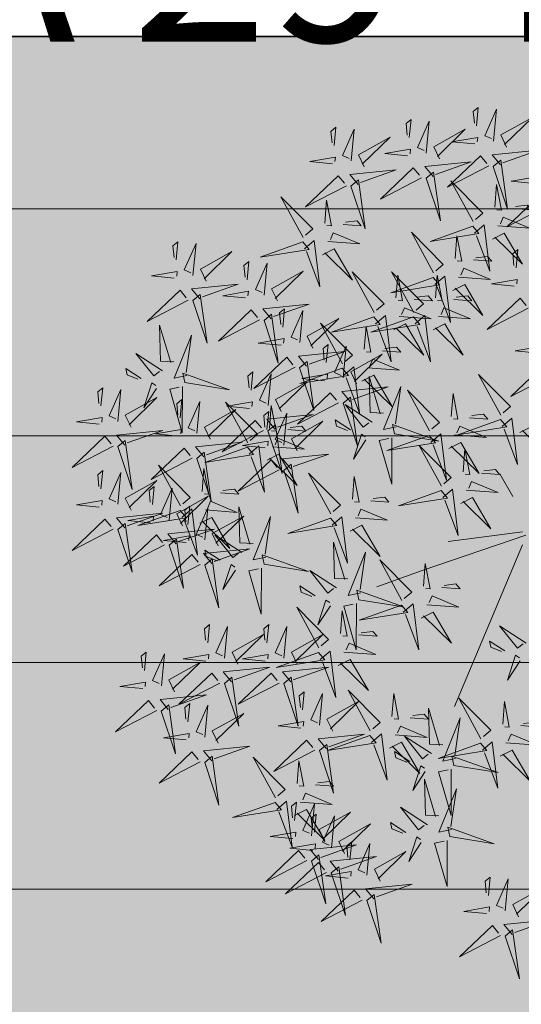
# Model space of a CAD drawing. Units: inches. Extents: x 1704 to 6393, y -157 to 1172.
# Tile 99 of 122: x 2561 to 2577, y 1001 to 1034. Entities that reach past the tile are written whole.
import ezdxf

# ---------------------------------------------------------------- set-up
doc = ezdxf.new("R2010")
doc.units = ezdxf.units.IN
doc.header["$MEASUREMENT"] = 0
for name, color, linetype, lineweight in [('A-ANNO-DIMS', 7, 'Continuous', 13), ('C-PROP', 7, 'Continuous', 35), ('L-DECK-PLNK-PATT', 250, 'Continuous', 13), ('L-shrub', 74, 'Continuous', 18), ('L-tree', 102, 'Continuous', 18)]:
    doc.layers.add(name, color=color, linetype=linetype, lineweight=lineweight)
doc.layers.add('L-DECK-PATT', color=35, linetype='Continuous', lineweight=13, true_color=0xa6725b)
doc.styles.get("Standard").update_dxf_attribs({"font": 'arial.ttf'})
doc.dimstyles.get("Standard").update_dxf_attribs({"dimtxt": 6, "dimasz": 2, "dimexe": 0.18, "dimexo": 0.0625, "dimgap": 0.09, "dimtad": 0, "dimtih": 1, "dimtoh": 1, "dimdec": 1, "dimzin": 0, "dimdsep": 46, "dimlunit": 3, "dimtxsty": 'Standard', "dimblk": 'ARCHTICK', "dimcen": 0.09, "dimadec": 0, "dimazin": 0, "dimtfac": 1, "dimtdec": 1, "dimtofl": 0, "dimtmove": 0, "dimatfit": 3, "dimfxl": 1, "dimtolj": 1, "dimtzin": 0, "dimarcsym": 0})

# ---------------------------------------------------------------- blocks, each defined once
blk = doc.blocks.new('bamboo')
blk.add_line((390, 162.3), (546.4, 218.1))
at = {"layer": 'L-shrub'}
for p, q in [((43.5, 73), (278.2, 631.2)), ((32.3, 39.5), (390, 162.3)), ((43.5, 28.4), (300.5, 61.9)), ((77, -94.4), (121.7, -172.6))]:
    blk.add_line(p, q, dxfattribs=at)
for points in [[(103.7, 1424.7), (54.4, 1572.3), (77.9, 1403.4), (103.7, 1424.7)], [(119.4, 1423.2), (261.4, 1496.7), (147.9, 1388.7), (126.6, 1414.5)], [(581.6, 1302), (532.2, 1449.6), (555.7, 1280.7), (581.6, 1302)], [(79.4, 1419.1), (107.8, 1384.6), (-52.4, 1368.4), (70.8, 1412)], [(597.3, 1300.4), (739.2, 1374), (625.7, 1265.9), (604.4, 1291.8)], [(57.7, 1357.7), (77.5, 1316.1), (-31.5, 1255.3), (64.8, 1349.1)], [(103.3, 1337.4), (92.8, 1227.4), (133.3, 1318.7), (110.4, 1328.8)], [(167.7, 1347.1), (246.3, 1339.5), (157.6, 1324.2), (159.1, 1340)], [(704.4, 1206.5), (655.1, 1354.1), (678.6, 1185.2), (704.4, 1206.5)], [(557.2, 1296.4), (585.7, 1261.9), (425.4, 1245.7), (548.6, 1289.3)], [(772.7, 1165.6), (723.3, 1313.2), (746.9, 1144.3), (772.7, 1165.6)], [(161.7, 1284.2), (155.7, 1221.3), (172.9, 1235.5), (168.8, 1275.6)], [(720.2, 1205), (862.1, 1278.5), (748.6, 1170.5), (727.3, 1196.4)], [(303.5, 1094), (304.2, 1253.9), (347.3, 1103.2), (314.4, 1096.3)], [(535.5, 1235), (555.3, 1193.4), (446.4, 1132.5), (542.6, 1226.4)], [(788.4, 1164.1), (930.3, 1237.6), (816.9, 1129.6), (795.5, 1155.5)], [(680.1, 1200.9), (708.6, 1166.4), (548.3, 1150.2), (671.5, 1193.8)], [(581.2, 1214.7), (570.7, 1104.6), (611.1, 1195.9), (588.3, 1206.1)], [(645.6, 1224.3), (724.2, 1216.7), (635.4, 1201.5), (637, 1217.2)], [(393.3, 1101.5), (436.5, 1167.6), (408.8, 1082), (395.6, 1090.6)], [(748.4, 1160), (776.8, 1125.5), (616.6, 1109.3), (739.8, 1152.9)], [(639.6, 1161.5), (633.5, 1098.6), (650.8, 1112.8), (646.7, 1152.8)], [(658.4, 1139.6), (678.2, 1098), (569.2, 1037.1), (665.5, 1130.9)], [(768.4, 1128.9), (847.1, 1121.3), (758.3, 1106.1), (759.8, 1121.8)], [(294.9, 1080.8), (141.2, 1105.5), (301.8, 1048), (294.9, 1080.8)], [(726.6, 1098.6), (746.5, 1057), (637.5, 996.2), (733.8, 1090)], [(704, 1119.3), (693.5, 1009.2), (734, 1100.5), (711.2, 1110.6)], [(830.7, 1007.8), (789.5, 987.1), (726.4, 1094.8), (822.2, 1000.5)], [(892.5, 987.3), (858.6, 958.2), (839.1, 1118), (885.2, 995.8)], [(288.5, 1056.7), (332.3, 1065.9), (272.3, 916.4), (290.8, 1045.7)], [(372, 1040), (464.6, 979.6), (402.5, 1057.8), (382.9, 1042.3)], [(446.2, 1067), (499.2, 1032.5), (494.6, 1054.4), (457.2, 1069.3)], [(762.4, 1066), (756.4, 1003.1), (773.6, 1017.3), (769.5, 1057.4)], [(772.3, 1078.4), (761.8, 968.3), (802.3, 1059.6), (779.4, 1069.7)], [(836.7, 1088), (915.3, 1080.4), (826.6, 1065.2), (828.1, 1080.9)], [(830.7, 1025.1), (824.7, 962.2), (841.9, 976.4), (837.8, 1016.5)], [(289.9, 848.6), (290.5, 1008.4), (333.6, 857.8), (300.8, 850.9)], [(332.8, 1008.9), (378.9, 1007.2), (382.3, 882.5), (343.8, 1011.2)], [(898.5, 963.1), (1045.1, 1015.5), (876.7, 988.5), (898.5, 963.1)], [(811.3, 961.7), (701, 970), (793.1, 931.4), (802.8, 954.4)], [(1141.3, 824.7), (1092, 972.3), (1115.5, 803.4), (1141.3, 824.7)], [(379.6, 856.1), (422.9, 922.2), (395.2, 836.5), (381.9, 845.1)], [(745.4, 783.8), (696, 931.4), (719.6, 762.5), (745.4, 783.8)], [(897.3, 947.3), (973.8, 807), (863.4, 918.2), (888.9, 940.1)], [(120.7, 803.3), (79.5, 782.6), (16.5, 890.3), (112.2, 796)], [(182.5, 782.8), (148.6, 753.6), (129.1, 913.5), (175.2, 791.2)], [(564.8, 755.5), (530.9, 726.4), (511.4, 886.2), (557.5, 764)], [(759.2, 902.3), (696.2, 907), (710.8, 890.1), (750.8, 895)], [(822.2, 897.5), (816.2, 818.8), (799.2, 907.2), (815, 906)], [(1157.1, 823.2), (1299, 896.7), (1185.5, 788.7), (1164.2, 814.6)], [(281.2, 835.4), (127.5, 860.1), (288.1, 802.6), (281.2, 835.4)], [(503, 776), (461.8, 755.3), (398.7, 863), (494.5, 768.7)], [(761.1, 782.3), (903, 855.8), (789.6, 747.8), (768.2, 773.7)], [(274.9, 811.2), (318.6, 820.4), (258.7, 670.9), (277.2, 800.3)], [(432.6, 821.6), (485.5, 787.1), (480.9, 808.9), (443.5, 823.9)], [(1117, 819.1), (1145.4, 784.6), (985.2, 768.4), (1108.4, 812)], [(188.6, 758.6), (335.2, 810.9), (166.8, 784), (188.6, 758.6)], [(358.3, 794.5), (451, 734.2), (388.8, 812.4), (369.3, 796.8)], [(570.9, 731.3), (717.4, 783.7), (549, 756.7), (570.9, 731.3)], [(1291.5, 647.4), (1242.1, 795), (1265.7, 626.1), (1291.5, 647.4)], [(101.4, 757.2), (-8.9, 765.5), (83.2, 726.9), (92.9, 749.9)], [(319.2, 763.5), (365.2, 761.8), (368.6, 637), (330.1, 765.8)], [(721.1, 778.2), (749.5, 743.7), (589.3, 727.5), (712.5, 771.1)], [(1095.3, 757.7), (1115.1, 716.2), (1006.1, 655.3), (1102.4, 749.1)], [(187.4, 742.8), (263.8, 602.4), (153.5, 713.7), (178.9, 735.5)], [(483.6, 729.9), (373.4, 738.2), (465.5, 699.6), (475.2, 722.6)], [(569.7, 715.5), (646.1, 575.2), (535.8, 686.4), (561.2, 708.3)], [(699.3, 716.8), (719.2, 675.2), (610.2, 614.4), (706.4, 708.2)], [(1140.9, 737.5), (1130.4, 627.4), (1170.9, 718.7), (1148, 728.8)], [(1205.3, 747.1), (1283.9, 739.5), (1195.2, 724.3), (1196.7, 740)], [(1307.2, 645.9), (1449.1, 719.5), (1335.7, 611.4), (1314.3, 637.3)], [(49.3, 697.7), (-13.7, 702.5), (0.8, 685.5), (40.8, 690.4)], [(112.3, 693), (106.3, 614.2), (89.3, 702.6), (105, 701.5)], [(745, 696.6), (734.5, 586.5), (774.9, 677.8), (752.1, 687.9)], [(809.4, 706.2), (888, 698.6), (799.3, 683.4), (800.8, 699.1)], [(868.3, 552), (818.9, 699.6), (842.4, 530.7), (868.3, 552)], [(1073.1, 552), (1023.7, 699.6), (1047.2, 530.7), (1073.1, 552)], [(1199.3, 684.2), (1193.3, 621.3), (1210.5, 635.5), (1206.4, 675.6)], [(431.6, 670.5), (368.6, 675.2), (383.1, 658.2), (423.1, 663.2)], [(494.6, 665.7), (488.6, 587), (471.6, 675.4), (487.3, 674.2)], [(803.4, 643.3), (797.4, 580.4), (814.6, 594.6), (810.5, 634.7)], [(884, 550.5), (1025.9, 624), (912.4, 516), (891.1, 541.8)], [(1088.8, 550.5), (1230.7, 624), (1117.2, 516), (1095.9, 541.8)], [(1267.2, 641.9), (1295.6, 607.4), (1135.4, 591.1), (1258.6, 634.8)], [(742.3, 469.2), (708.4, 440), (688.9, 599.9), (735, 477.6)], [(1245.4, 580.5), (1265.3, 538.9), (1156.3, 478), (1252.6, 571.9)], [(680.5, 489.6), (639.3, 469), (576.2, 576.7), (672, 482.3)], [(843.9, 546.4), (872.4, 511.9), (712.1, 495.7), (835.3, 539.3)], [(1048.7, 546.4), (1077.2, 511.9), (916.9, 495.7), (1040.1, 539.3)], [(1291.1, 560.2), (1280.6, 450.1), (1321.1, 541.4), (1298.2, 551.6)], [(1355.5, 569.8), (1434.1, 562.2), (1345.4, 547), (1346.9, 562.7)], [(52, 474.3), (95.2, 540.4), (67.5, 454.7), (54.3, 463.3)], [(748.4, 444.9), (894.9, 497.3), (726.5, 470.3), (748.4, 444.9)], [(822.2, 485), (842, 443.4), (733.1, 382.6), (829.3, 476.4)], [(1027, 485), (1046.8, 443.4), (937.9, 382.6), (1034.1, 476.4)], [(1349.5, 506.9), (1343.5, 444), (1360.7, 458.2), (1356.6, 498.3)], [(661.1, 443.6), (550.9, 451.8), (643, 413.2), (652.6, 436.3)], [(867.9, 464.7), (857.4, 354.7), (897.8, 446), (875, 456.1)], [(932.3, 474.4), (1010.9, 466.8), (922.2, 451.6), (923.7, 467.3)], [(1072.7, 464.7), (1062.1, 354.7), (1102.6, 446), (1079.8, 456.1)], [(1137.1, 474.4), (1215.7, 466.8), (1126.9, 451.6), (1128.4, 467.3)], [(30.7, 412.7), (123.3, 352.4), (61.2, 430.6), (41.6, 415)], [(104.9, 439.8), (157.9, 405.3), (153.3, 427.1), (115.9, 442.1)], [(393.8, 326), (352.6, 305.3), (289.5, 413), (385.3, 318.7)], [(455.6, 305.5), (421.7, 276.4), (402.2, 436.3), (448.3, 314)], [(617.5, 275.9), (618.2, 435.7), (661.3, 285.1), (628.5, 278.2)], [(747.2, 429.2), (823.6, 288.8), (713.3, 400), (738.7, 421.9)], [(926.3, 411.5), (920.3, 348.6), (937.5, 362.8), (933.4, 402.9)], [(1131.1, 411.5), (1125, 348.6), (1142.3, 362.8), (1138.2, 402.9)], [(609.1, 384.1), (546.1, 388.8), (560.6, 371.9), (600.6, 376.8)], [(672.1, 379.4), (666.1, 300.6), (649, 389), (664.8, 387.8)], [(707.3, 283.4), (750.5, 349.5), (722.8, 263.8), (709.6, 272.4)], [(461.7, 281.3), (608.2, 333.7), (439.8, 306.7), (461.7, 281.3)], [(945.2, 153.2), (945.8, 313), (988.9, 162.4), (956.1, 155.5)], [(374.4, 279.9), (264.1, 288.2), (356.3, 249.6), (365.9, 272.6)], [(608.9, 262.7), (455.2, 287.4), (615.8, 229.9), (608.9, 262.7)], [(1141.3, 142.9), (1092, 290.5), (1115.5, 121.6), (1141.3, 142.9)], [(460.4, 265.6), (536.9, 125.2), (426.5, 236.4), (452, 258.3)], [(602.5, 238.5), (646.3, 247.7), (586.3, 98.2), (604.8, 227.6)], [(686, 221.8), (778.6, 161.5), (716.5, 239.7), (696.9, 224.1)], [(760.2, 248.9), (813.2, 214.4), (808.6, 236.2), (771.2, 251.2)], [(322.4, 220.5), (259.3, 225.2), (273.9, 208.3), (313.9, 213.2)], [(385.4, 215.7), (379.4, 137), (362.3, 225.4), (378.1, 224.2)], [(1035, 160.6), (1078.2, 226.8), (1050.5, 141.1), (1037.3, 149.7)], [(1157.1, 141.4), (1299, 214.9), (1185.5, 106.9), (1164.2, 132.8)], [(1264.2, 74.7), (1214.8, 222.3), (1238.4, 53.4), (1264.2, 74.7)], [(646.8, 190.8), (692.9, 189.1), (696.3, 64.3), (657.8, 193.1)], [(701.3, 5.5), (667.4, -23.6), (647.9, 136.3), (694, 14)], [(936.5, 139.9), (782.9, 164.7), (943.4, 107.2), (936.5, 139.9)], [(1117, 137.3), (1145.4, 102.8), (985.2, 86.6), (1108.4, 130.2)], [(1279.9, 73.2), (1421.8, 146.8), (1308.4, 38.7), (1287, 64.6)], [(1441.7, 20.2), (1392.3, 167.8), (1415.9, -1.1), (1441.7, 20.2)], [(639.5, 26), (598.3, 5.3), (535.3, 113), (631, 18.7)], [(930.2, 115.8), (973.9, 125), (914, -24.5), (932.5, 104.9)], [(1013.6, 99.1), (1106.3, 38.8), (1044.2, 116.9), (1024.6, 101.4)], [(1087.9, 126.1), (1140.9, 91.6), (1136.3, 113.5), (1098.9, 128.4)], [(1220.1, -21.7), (1186.2, -50.9), (1166.7, 109), (1212.8, -13.3)], [(974.5, 68.1), (1020.5, 66.3), (1023.9, -58.4), (985.4, 70.4)], [(1095.3, 76), (1115.1, 34.4), (1006.1, -26.5), (1102.4, 67.3)], [(1158.3, -1.3), (1117.1, -21.9), (1054.1, 85.8), (1149.8, -8.5)], [(1239.9, 69.2), (1268.3, 34.7), (1108.1, 18.4), (1231.3, 62.1)], [(1457.4, 18.7), (1599.3, 92.2), (1485.9, -15.8), (1464.5, 10)], [(319, -89.9), (285.1, -119.1), (265.6, 40.8), (311.8, -81.4)], [(1140.9, 55.7), (1130.4, -54.4), (1170.9, 36.9), (1148, 47)], [(1205.3, 65.3), (1283.9, 57.7), (1195.2, 42.5), (1196.7, 58.2)], [(257.2, -69.4), (216.1, -90.1), (153, 17.6), (248.8, -76.7)], [(707.4, -18.7), (854, 33.7), (685.6, 6.7), (707.4, -18.7)], [(1218.1, 7.8), (1238, -33.8), (1129, -94.7), (1225.2, -0.8)], [(1199.3, 2.4), (1193.3, -60.5), (1210.5, -46.3), (1206.4, -6.2)], [(1226.2, -46), (1372.8, 6.4), (1204.4, -20.6), (1226.2, -46)], [(1417.4, 14.6), (1445.8, -19.9), (1285.6, -36.1), (1408.7, 7.5)], [(620.2, -20.1), (509.9, -11.8), (602, -50.4), (611.7, -27.3)], [(1263.8, -12.5), (1253.3, -122.6), (1293.7, -31.3), (1270.9, -21.1)], [(1328.2, -2.9), (1406.8, -10.5), (1318.1, -25.7), (1319.6, -10)], [(325.1, -114.1), (471.7, -61.8), (303.3, -88.7), (325.1, -114.1)], [(706.2, -34.4), (782.6, -174.8), (672.3, -63.6), (697.7, -41.7)], [(868.3, -184.3), (818.9, -36.7), (842.4, -205.6), (868.3, -184.3)], [(1139, -47.3), (1028.7, -39.1), (1120.8, -77.6), (1130.5, -54.6)], [(1225, -61.7), (1301.4, -202.1), (1191.1, -90.8), (1216.5, -69)], [(1395.6, -46.8), (1415.5, -88.4), (1306.5, -149.2), (1402.7, -55.4)], [(1322.2, -65.8), (1316.2, -128.7), (1333.4, -114.5), (1329.3, -74.4)], [(1441.3, -67.1), (1430.8, -177.1), (1471.2, -85.8), (1448.4, -75.7)], [(1505.7, -57.4), (1584.3, -65), (1495.6, -80.2), (1497.1, -64.5)], [(568.1, -79.5), (505.1, -74.8), (519.6, -91.7), (559.6, -86.8)], [(631.1, -84.2), (625.1, -163), (608.1, -74.6), (623.8, -75.8)], [(1168.6, -225.3), (1119.3, -77.6), (1142.8, -246.6), (1168.6, -225.3)], [(1149.9, -111.5), (1143.9, -190.3), (1126.9, -101.9), (1142.6, -103)], [(237.9, -115.5), (127.6, -107.2), (219.7, -145.8), (229.4, -122.8)], [(323.9, -129.9), (400.4, -270.3), (290, -159), (315.4, -137.2)], [(926.2, -219.4), (885, -240.1), (822, -132.4), (917.7, -226.7)], [(884, -185.9), (1025.9, -112.3), (912.4, -220.4), (891.1, -194.5)], [(988, -239.9), (954.1, -269), (934.6, -109.2), (980.8, -231.4)], [(1086.9, -106.8), (1023.9, -102.1), (1038.4, -119), (1078.4, -114.1)], [(1441.7, -266.2), (1392.3, -118.6), (1415.9, -287.5), (1441.7, -266.2)], [(1499.7, -120.3), (1493.7, -183.2), (1510.9, -169), (1506.8, -128.9)], [(248.8, -179.7), (242.8, -258.4), (225.8, -170), (241.6, -171.2)], [(360, -280.8), (326.1, -310), (306.6, -150.1), (352.7, -272.3)], [(494.6, -296.8), (495.3, -137), (538.4, -287.6), (505.6, -294.5)], [(1184.4, -226.8), (1326.3, -153.2), (1212.8, -261.3), (1191.5, -235.4)], [(185.8, -175), (122.8, -170.2), (137.4, -187.2), (177.4, -182.3)], [(298.2, -260.3), (257, -281), (193.9, -173.3), (289.7, -267.6)], [(843.9, -189.9), (872.4, -224.4), (712.1, -240.6), (835.3, -197)], [(922.9, -320.7), (873.5, -173.1), (897.1, -342), (922.9, -320.7)], [(1457.4, -267.7), (1599.3, -194.1), (1485.9, -302.2), (1464.5, -276.3)], [(52.5, -314.9), (11.3, -335.6), (-51.8, -227.9), (44, -322.2)], [(114.3, -335.4), (80.4, -364.5), (60.9, -204.6), (107, -326.9)], [(584.4, -289.3), (627.6, -223.2), (600, -308.9), (586.7, -300.3)], [(994.1, -264.1), (1140.7, -211.8), (972.3, -238.7), (994.1, -264.1)], [(1144.3, -230.8), (1172.7, -265.3), (1012.5, -281.6), (1135.7, -237.9)], [(366.1, -305), (512.7, -252.7), (344.3, -279.6), (366.1, -305)], [(663.5, -416.2), (614.1, -268.5), (637.6, -437.5), (663.5, -416.2)], [(822.2, -251.3), (842, -292.9), (733.1, -353.8), (829.3, -259.9)], [(906.9, -265.5), (796.6, -257.2), (888.7, -295.8), (898.4, -272.8)], [(867.9, -271.6), (857.4, -381.7), (897.8, -290.4), (875, -280.2)], [(932.3, -262), (1010.9, -269.6), (922.2, -284.8), (923.7, -269.1)], [(938.6, -322.2), (1080.5, -248.7), (967.1, -356.7), (945.7, -330.8)], [(1417.4, -271.7), (1445.8, -306.2), (1285.6, -322.5), (1408.7, -278.8)], [(278.8, -306.4), (168.6, -298.1), (260.7, -336.7), (270.4, -313.7)], [(486, -310), (332.3, -285.3), (492.9, -342.8), (486, -310)], [(992.9, -279.9), (1069.3, -420.3), (959, -309), (984.4, -287.2)], [(1122.6, -292.2), (1142.4, -333.8), (1033.4, -394.7), (1129.7, -300.8)], [(1232.6, -302.9), (1311.2, -310.5), (1222.5, -325.7), (1224, -310)], [(120.3, -359.6), (266.9, -307.2), (98.5, -334.2), (120.3, -359.6)], [(364.9, -320.8), (441.3, -461.2), (331, -349.9), (356.4, -328.1)], [(479.7, -334.2), (523.4, -325), (463.5, -474.5), (482, -345.1)], [(563.1, -350.9), (655.8, -411.2), (593.6, -333), (574, -348.6)], [(637.4, -323.8), (690.3, -358.3), (685.7, -336.5), (648.3, -321.5)], [(898.6, -326.3), (927, -360.8), (766.8, -377), (889.9, -333.4)], [(854.8, -325), (791.8, -320.2), (806.4, -337.2), (846.3, -332.2)], [(917.8, -329.7), (911.8, -408.4), (894.8, -320), (910.5, -321.2)], [(926.3, -324.9), (920.3, -387.8), (937.5, -373.5), (933.4, -333.5)], [(1168.2, -312.5), (1157.7, -422.6), (1198.2, -331.3), (1175.3, -321.1)], [(1218.2, -474.1), (1218.9, -314.2), (1262, -464.9), (1229.2, -471.8)], [(1395.6, -333.1), (1415.5, -374.7), (1306.5, -435.6), (1402.7, -341.7)], [(226.8, -365.9), (163.8, -361.1), (178.3, -378.1), (218.3, -373.2)], [(289.8, -370.6), (283.8, -449.3), (266.8, -360.9), (282.5, -362.1)], [(679.2, -417.7), (821.1, -344.1), (707.7, -452.2), (686.3, -426.3)], [(1226.6, -365.8), (1220.6, -428.7), (1237.8, -414.5), (1233.7, -374.4)], [(1441.3, -353.4), (1430.8, -463.5), (1471.2, -372.2), (1448.4, -362)], [(1505.7, -343.8), (1584.3, -351.4), (1495.6, -366.6), (1497.1, -350.9)], [(119.1, -375.3), (195.6, -515.7), (85.2, -404.5), (110.7, -382.6)], [(598.6, -492.1), (557.4, -512.8), (494.3, -405.1), (590.1, -499.4)], [(524, -381.9), (570, -383.6), (573.4, -508.4), (534.9, -379.6)], [(660.4, -512.6), (626.5, -541.8), (607, -381.9), (653.1, -504.2)], [(813.7, -538.9), (764.3, -391.3), (787.8, -560.2), (813.7, -538.9)], [(876.8, -387.7), (896.6, -429.3), (787.7, -490.1), (883.9, -396.3)], [(922.5, -407.9), (912, -518), (952.4, -426.7), (929.6, -416.6)], [(986.9, -398.3), (1065.5, -405.9), (976.8, -421.1), (978.3, -405.4)], [(1308, -466.6), (1351.2, -400.5), (1323.6, -486.2), (1310.3, -477.5)], [(1499.7, -406.7), (1493.7, -469.6), (1510.9, -455.4), (1506.8, -415.3)], [(-58, -513.1), (83.9, -439.6), (-29.6, -547.6), (-50.9, -521.7)], [(639.2, -421.7), (667.6, -456.2), (507.4, -472.5), (630.5, -428.8)], [(829.4, -540.4), (971.3, -466.8), (857.8, -574.9), (836.5, -549)], [(980.9, -461.2), (974.9, -524.1), (992.1, -509.9), (988, -469.8)], [(1209.6, -487.3), (1055.9, -462.6), (1216.5, -520.1), (1209.6, -487.3)], [(617.4, -483.1), (637.2, -524.7), (528.3, -585.6), (624.5, -491.7)], [(666.4, -536.8), (813, -484.5), (644.6, -511.4), (666.4, -536.8)], [(663.1, -503.4), (652.6, -613.5), (693, -522.2), (670.2, -512)], [(727.5, -493.8), (806.1, -501.4), (717.4, -516.6), (718.9, -500.9)], [(1203.3, -511.5), (1247, -502.3), (1187.1, -651.7), (1205.5, -522.4)], [(1361, -501.1), (1413.9, -535.6), (1409.3, -513.8), (1371.9, -498.8)], [(579.2, -538.2), (468.9, -529.9), (561.1, -568.5), (570.7, -545.5)], [(1286.7, -528.1), (1379.3, -588.5), (1317.2, -510.3), (1297.6, -525.8)], [(414.6, -689.9), (380.7, -719), (361.2, -559.2), (407.3, -681.4)], [(551.1, -689.9), (517.2, -719), (497.7, -559.2), (543.9, -681.4)], [(665.2, -552.6), (741.7, -693), (631.3, -581.7), (656.8, -559.9)], [(789.3, -544.5), (817.8, -578.9), (657.5, -595.2), (780.7, -551.6)], [(721.5, -556.7), (715.5, -619.6), (732.7, -605.4), (728.6, -565.3)], [(936.5, -702.5), (887.2, -554.9), (910.7, -723.8), (936.5, -702.5)], [(1247.5, -559.2), (1293.6, -560.9), (1297, -685.7), (1258.5, -556.9)], [(-9.8, -589.2), (68.8, -596.8), (-19.9, -612), (-18.4, -596.3)], [(352.8, -669.4), (311.6, -690.1), (248.5, -582.4), (344.3, -676.7)], [(489.3, -669.4), (448.2, -690.1), (385.1, -582.4), (480.9, -676.7)], [(527.1, -597.7), (464.1, -593), (478.7, -609.9), (518.7, -605)], [(590.2, -602.4), (584.1, -681.2), (567.1, -592.8), (582.9, -593.9)], [(767.6, -605.8), (787.4, -647.4), (678.5, -708.3), (774.7, -614.5)], [(813.3, -626.1), (802.7, -736.2), (843.2, -644.9), (820.4, -634.7)], [(877.7, -616.5), (956.3, -624.1), (867.5, -639.3), (869, -623.6)], [(952.3, -704), (1094.2, -630.5), (980.7, -738.5), (959.4, -712.7)], [(1182.3, -770.7), (1132.9, -623.1), (1156.5, -792), (1182.3, -770.7)], [(23.9, -744.9), (165.8, -671.4), (52.3, -779.4), (31, -753.6)], [(420.7, -714.1), (567.3, -661.7), (398.9, -688.7), (420.7, -714.1)], [(557.2, -714.1), (703.8, -661.7), (535.4, -688.7), (557.2, -714.1)], [(871.6, -679.4), (865.6, -742.3), (882.9, -728.1), (878.8, -688)], [(333.5, -715.5), (223.2, -707.2), (315.3, -745.8), (325, -722.8)], [(346.4, -826.2), (312.4, -855.4), (293, -695.5), (339.1, -817.8)], [(470, -715.5), (359.7, -707.2), (451.8, -745.8), (461.5, -722.8)], [(912.2, -708.1), (940.6, -742.6), (780.4, -758.8), (903.6, -715.2)], [(1198, -772.2), (1339.9, -698.7), (1226.5, -806.7), (1205.1, -780.8)], [(284.5, -805.8), (243.4, -826.4), (180.3, -718.7), (276.1, -813.1)], [(419.5, -729.9), (495.9, -870.2), (385.6, -759), (411, -737.1)], [(556, -729.9), (632.4, -870.2), (522.1, -759), (547.5, -737.1)], [(281.4, -774.9), (218.4, -770.2), (232.9, -787.1), (272.9, -782.2)], [(344.4, -779.7), (338.4, -858.4), (321.4, -770), (337.1, -771.2)], [(417.9, -774.9), (354.9, -770.2), (369.5, -787.1), (409.4, -782.2)], [(480.9, -779.7), (474.9, -858.4), (457.9, -770), (473.7, -771.2)], [(890.5, -769.5), (910.3, -811.1), (801.3, -871.9), (897.6, -778.1)], [(1000.5, -780.1), (1079.1, -787.7), (990.4, -802.9), (991.9, -787.2)], [(1158, -776.3), (1186.4, -810.8), (1026.2, -827), (1149.3, -783.4)], [(352.4, -850.5), (499, -798.1), (330.6, -825.1), (352.4, -850.5)], [(936.1, -789.8), (925.6, -899.8), (966.1, -808.5), (943.2, -798.4)], [(72.2, -821), (150.8, -828.6), (62, -843.8), (63.5, -828.1)], [(265.2, -851.8), (154.9, -843.6), (247, -882.2), (256.7, -859.1)], [(735.1, -928.5), (693.9, -949.2), (630.8, -841.5), (726.6, -935.8)], [(796.9, -949), (763, -978.1), (743.5, -818.2), (789.6, -940.5)], [(994.5, -843), (988.5, -905.9), (1005.7, -891.7), (1001.6, -851.6)], [(1136.2, -837.6), (1156, -879.2), (1047.1, -940.1), (1143.3, -846.3)], [(1246.3, -848.3), (1324.9, -855.9), (1236.2, -871.1), (1237.7, -855.4)], [(66.1, -883.9), (60.1, -946.8), (77.4, -932.6), (73.3, -892.5)], [(209.8, -1003.5), (175.9, -1032.7), (156.4, -872.8), (202.6, -995)], [(351.2, -866.2), (427.7, -1006.6), (317.3, -895.4), (342.8, -873.5)], [(1181.9, -857.9), (1171.4, -968), (1211.8, -876.7), (1189, -866.6)], [(148, -983), (106.8, -1003.7), (43.8, -896), (139.5, -990.3)], [(213.1, -911.3), (150.1, -906.6), (164.7, -923.5), (204.7, -918.6)], [(276.1, -916), (270.1, -994.8), (253.1, -906.4), (268.9, -907.6)], [(1240.3, -911.2), (1234.3, -974.1), (1251.5, -959.9), (1247.4, -919.8)], [(803, -973.2), (949.5, -920.8), (781.1, -947.8), (803, -973.2)], [(215.9, -1027.7), (362.5, -975.4), (194.1, -1002.3), (215.9, -1027.7)], [(715.7, -974.6), (605.5, -966.3), (697.6, -1004.9), (707.3, -981.8)], [(636.2, -1166.1), (586.8, -1018.5), (610.3, -1187.4), (636.2, -1166.1)], [(801.8, -988.9), (878.2, -1129.3), (767.9, -1018.1), (793.3, -996.2)], [(-44.4, -1099.5), (97.5, -1025.9), (-15.9, -1134), (-37.3, -1108.1)], [(128.7, -1029.1), (18.4, -1020.8), (110.5, -1059.4), (120.2, -1036.4)], [(214.7, -1043.5), (291.1, -1183.9), (180.8, -1072.6), (206.2, -1050.8)], [(376.8, -1193.4), (327.4, -1045.8), (350.9, -1214.7), (376.8, -1193.4)], [(663.7, -1034), (600.7, -1029.3), (615.2, -1046.2), (655.2, -1041.3)], [(726.7, -1038.7), (720.7, -1117.5), (703.7, -1029.1), (719.4, -1030.3)], [(76.6, -1088.6), (13.6, -1083.8), (28.1, -1100.8), (68.1, -1095.8)], [(144.7, -1234.3), (95.3, -1086.7), (118.8, -1255.6), (144.7, -1234.3)], [(139.6, -1093.3), (133.6, -1172), (116.6, -1083.6), (132.3, -1084.8)], [(392.5, -1194.9), (534.4, -1121.4), (420.9, -1229.4), (399.6, -1203.5)], [(651.9, -1167.6), (793.8, -1094.1), (680.3, -1202.1), (659, -1176.3)], [(3.9, -1175.6), (82.5, -1183.2), (-6.2, -1198.4), (-4.7, -1182.7)], [(160.4, -1235.8), (302.3, -1162.3), (188.8, -1270.3), (167.5, -1244.4)], [(611.8, -1171.7), (640.3, -1206.2), (480.1, -1222.4), (603.2, -1178.8)], [(352.4, -1199), (380.9, -1233.5), (220.7, -1249.7), (343.8, -1206.1)], [(120.3, -1239.9), (148.8, -1274.4), (-11.4, -1290.6), (111.7, -1247)], [(590.1, -1233.1), (609.9, -1274.7), (501, -1335.5), (597.2, -1241.7)], [(635.8, -1253.4), (625.3, -1363.4), (665.7, -1272.1), (642.9, -1262)], [(700.2, -1243.7), (778.8, -1251.3), (690.1, -1266.6), (691.6, -1250.8)], [(330.7, -1260.4), (350.5, -1301.9), (241.6, -1362.8), (337.8, -1269)], [(376.4, -1280.6), (365.9, -1390.7), (406.3, -1299.4), (383.5, -1289.3)], [(440.8, -1271), (519.4, -1278.6), (430.7, -1293.8), (432.2, -1278.1)], [(98.6, -1301.3), (118.4, -1342.9), (9.5, -1403.7), (105.7, -1309.9)], [(144.3, -1321.5), (133.8, -1431.6), (174.2, -1340.3), (151.4, -1330.2)], [(208.7, -1311.9), (287.3, -1319.5), (198.6, -1334.7), (200.1, -1319)], [(694.2, -1306.6), (688.2, -1369.5), (705.4, -1355.3), (701.3, -1315.3)], [(434.8, -1333.9), (428.8, -1396.8), (446, -1382.6), (441.9, -1342.5)], [(202.7, -1374.8), (196.7, -1437.7), (213.9, -1423.5), (209.8, -1383.4)]]:
    blk.add_lwpolyline(points, dxfattribs=at)
blk = doc.blocks.new('_ArchTick')
at = {"color": 0, "linetype": 'ByBlock', "const_width": 0.15}
blk.add_lwpolyline([(-0.5, -0.5), (0.5, 0.5)], dxfattribs=at)
blk = doc.blocks.new('*D88')
at = {"layer": 'A-ANNO-DIMS', "color": 0, "lineweight": -2, "transparency": 16777216}
for p, q in [((2596.639, 1031.77), (2596.639, 1036.222)), ((2625.54, 1031.77), (2625.54, 1036.222)), ((2596.639, 1036.042), (2594.639, 1036.042)), ((2625.54, 1036.042), (2596.639, 1036.042))]:
    blk.add_line(p, q, dxfattribs=at)
at = {"layer": 'Defpoints', "color": 0, "lineweight": -3, "transparency": 16777216}
for p in [(2596.639, 1036.042), (2596.639, 1031.707), (2625.54, 1031.707)]:
    blk.add_point(p, dxfattribs=at)
at = {"layer": 'A-ANNO-DIMS', "color": 0, "lineweight": -2, "transparency": 16777216, "xscale": 2, "yscale": 2, "zscale": 2, "rotation": 180}
blk.add_blockref('_ArchTick', (2596.639, 1036.042), dxfattribs=at)
at = {"layer": 'A-ANNO-DIMS', "color": 0, "lineweight": -2, "transparency": 16777216, "xscale": 2, "yscale": 2, "zscale": 2}
blk.add_blockref('_ArchTick', (2625.54, 1036.042), dxfattribs=at)
at = {"layer": 'A-ANNO-DIMS', "color": 0, "transparency": 16777216, "insert": (2560.165, 1036.042), "char_height": 6, "attachment_point": 5}
blk.add_mtext('\\A1;SHRUB A 29 TYP.', dxfattribs=at)
blk = doc.blocks.new('*D92')
at = {"layer": 'A-ANNO-DIMS', "color": 0, "lineweight": -2, "transparency": 16777216}
for p, q in [((2073.349, 895.275), (2073.349, 1105.287)), ((2605.349, 895.275), (2605.349, 1105.287)), ((2073.349, 1105.107), (2332.661, 1105.107)), ((2605.349, 1105.107), (2346.036, 1105.107))]:
    blk.add_line(p, q, dxfattribs=at)
at = {"layer": 'Defpoints', "color": 0, "lineweight": -3, "transparency": 16777216}
for p in [(2605.349, 1105.107), (2073.349, 895.213), (2605.349, 895.213)]:
    blk.add_point(p, dxfattribs=at)
at = {"layer": 'A-ANNO-DIMS', "color": 0, "lineweight": -2, "transparency": 16777216, "xscale": 2, "yscale": 2, "zscale": 2, "rotation": 180}
blk.add_blockref('_ArchTick', (2073.349, 1105.107), dxfattribs=at)
at = {"layer": 'A-ANNO-DIMS', "color": 0, "lineweight": -2, "transparency": 16777216, "xscale": 2, "yscale": 2, "zscale": 2}
blk.add_blockref('_ArchTick', (2605.349, 1105.107), dxfattribs=at)
at = {"layer": 'A-ANNO-DIMS', "color": 0, "transparency": 16777216, "insert": (2339.349, 1105.107), "char_height": 6, "attachment_point": 5}
blk.add_mtext('\\A1;532', dxfattribs=at)
blk = doc.blocks.new('*D103')
at = {"layer": 'A-ANNO-DIMS', "color": 0, "lineweight": -2, "transparency": 16777216}
for p, q in [((2551.349, 711.275), (2551.349, 1105.287)), ((2597.349, 711.275), (2597.349, 1105.287)), ((2551.349, 1105.107), (2569.842, 1105.107)), ((2597.349, 1105.107), (2578.855, 1105.107))]:
    blk.add_line(p, q, dxfattribs=at)
at = {"layer": 'Defpoints', "color": 0, "lineweight": -3, "transparency": 16777216}
for p in [(2597.349, 1105.107), (2551.349, 711.213), (2597.349, 711.213)]:
    blk.add_point(p, dxfattribs=at)
at = {"layer": 'A-ANNO-DIMS', "color": 0, "lineweight": -2, "transparency": 16777216, "xscale": 2, "yscale": 2, "zscale": 2, "rotation": 180}
blk.add_blockref('_ArchTick', (2551.349, 1105.107), dxfattribs=at)
at = {"layer": 'A-ANNO-DIMS', "color": 0, "lineweight": -2, "transparency": 16777216, "xscale": 2, "yscale": 2, "zscale": 2}
blk.add_blockref('_ArchTick', (2597.349, 1105.107), dxfattribs=at)
at = {"layer": 'A-ANNO-DIMS', "color": 0, "transparency": 16777216, "insert": (2574.349, 1105.107), "char_height": 6, "attachment_point": 5}
blk.add_mtext('\\A1;46', dxfattribs=at)

msp = doc.modelspace()

# ---------------------------------------------------------------- hatches: boundary and pattern name
at = {"layer": 'L-DECK-PATT', "transparency": 33554544}
h = msp.add_hatch(color=256, dxfattribs=at)
h.dxf.hatch_style = 1
h.paths.add_polyline_path([(2329.589, 1033.213), (2065.589, 1033.213), (2065.589, 895.213), (2167.349, 895.213), (2263.349, 895.213), (2263.349, 903.213), (2273.349, 903.213), (2273.349, 895.213), (2329.589, 895.213)])
h.paths.add_polyline_path([(2664.349, 1033.213), (2333.589, 1033.213), (2333.589, 895.213), (2465.349, 895.213), (2469.181, 895.213), (2470.482, 895.213), (2508.215, 895.213), (2509.516, 895.213), (2513.349, 895.213), (2533.349, 895.213), (2581.349, 895.213), (2605.349, 895.213), (2664.349, 895.213)])
h.paths.add_polyline_path([(2333.589, 1033.213), (2329.589, 1033.213), (2329.589, 895.213), (2333.589, 895.213)])
at = {"layer": 'L-DECK-PLNK-PATT'}
h = msp.add_hatch(dxfattribs=at)
h.set_pattern_fill('LINE', color=256, scale=60)
h.paths.add_polyline_path([(2329.589, 1033.213), (2065.589, 1033.213), (2065.589, 895.213), (2167.349, 895.213), (2263.349, 895.213), (2263.349, 903.213), (2273.349, 903.213), (2273.349, 895.213), (2329.589, 895.213)])
h.paths.add_polyline_path([(2664.349, 1033.213), (2333.589, 1033.213), (2333.589, 895.213), (2465.349, 895.213), (2469.181, 895.213), (2470.482, 895.213), (2508.215, 895.213), (2509.516, 895.213), (2513.349, 895.213), (2533.349, 895.213), (2581.349, 895.213), (2605.349, 895.213), (2664.349, 895.213)])
h.paths.add_polyline_path([(2333.589, 1033.213), (2329.589, 1033.213), (2329.589, 895.213), (2333.589, 895.213)])

# ---------------------------------------------------------------- linework, layer by layer
at = {"layer": 'C-PROP'}
msp.add_line((2723.349, 1033.213), (1898.349, 1033.213), dxfattribs=at)

# ---------------------------------------------------------------- block references
at = {"layer": 'L-tree', "xscale": 0.0095734028514679, "yscale": 0.0095734028514679, "zscale": 0.0095734028514679, "rotation": 180}
msp.add_blockref('bamboo', (2577.692, 1017.096), dxfattribs=at)

# ---------------------------------------------------------------- dimensions: what is measured, and where the dimension line sits
at = {"layer": 'A-ANNO-DIMS'}
for base, p1, p2, picture, middle in [((2605.349, 1105.107), (2073.349, 895.213), (2605.349, 895.213), '*D92', (2339.349, 1105.107)), ((2597.349, 1105.107), (2551.349, 711.213), (2597.349, 711.213), '*D103', (2574.349, 1105.107))]:
    dim = msp.add_linear_dim(base=base, p1=p1, p2=p2, dimstyle='Standard', override={"dimdec": 0, "dimlfac": 1, "dimrnd": 0, "dimzin": 0, "dimdsep": 46, "dimlunit": 2}, dxfattribs=at)
    dim.commit()
    dim.dimension.update_dxf_attribs({"geometry": picture, "text_midpoint": middle})
dim = msp.add_linear_dim(base=(2596.639, 1036.042), p1=(2625.54, 1031.707), p2=(2596.639, 1031.707), angle=180, text='SHRUB A <> TYP.', dimstyle='Standard', override={"dimdec": 0, "dimlfac": 1, "dimrnd": 0, "dimzin": 0, "dimdsep": 46, "dimlunit": 2}, dxfattribs=at)
dim.commit()
dim.dimension.update_dxf_attribs({"geometry": '*D88', "text_midpoint": (2560.165, 1036.042)})

doc.saveas('drawing.dxf')
